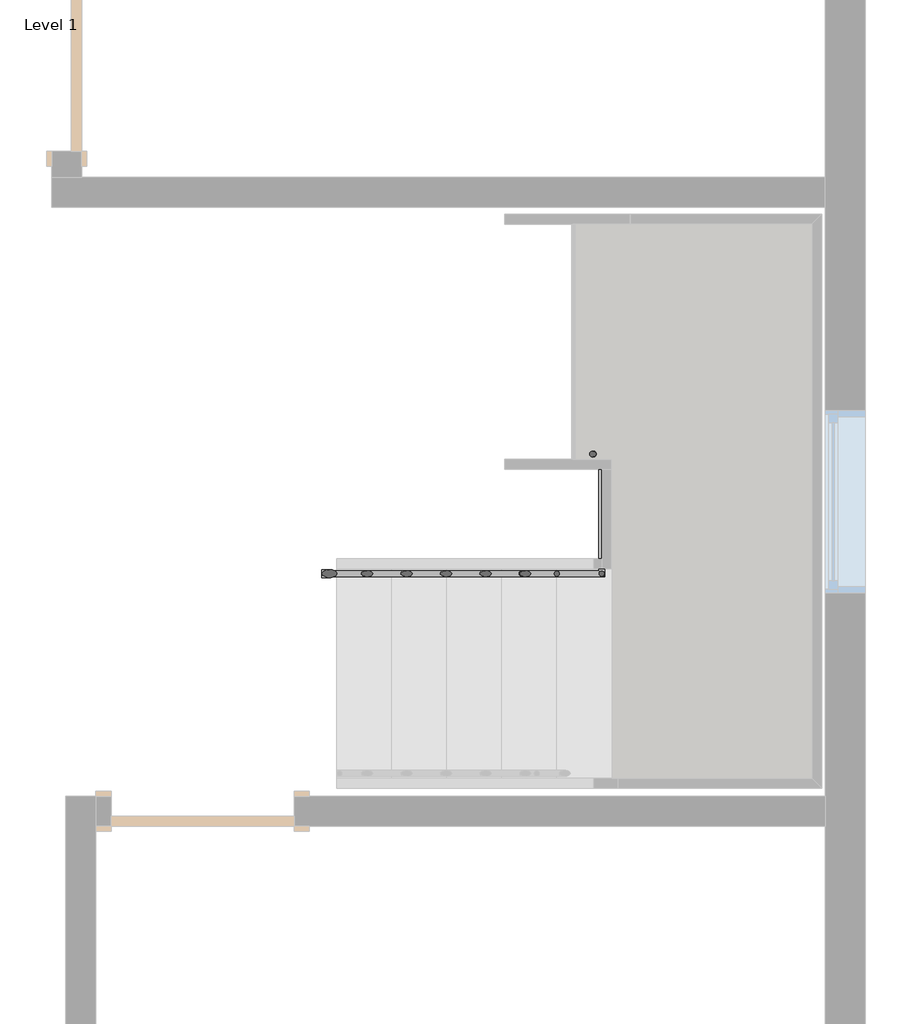
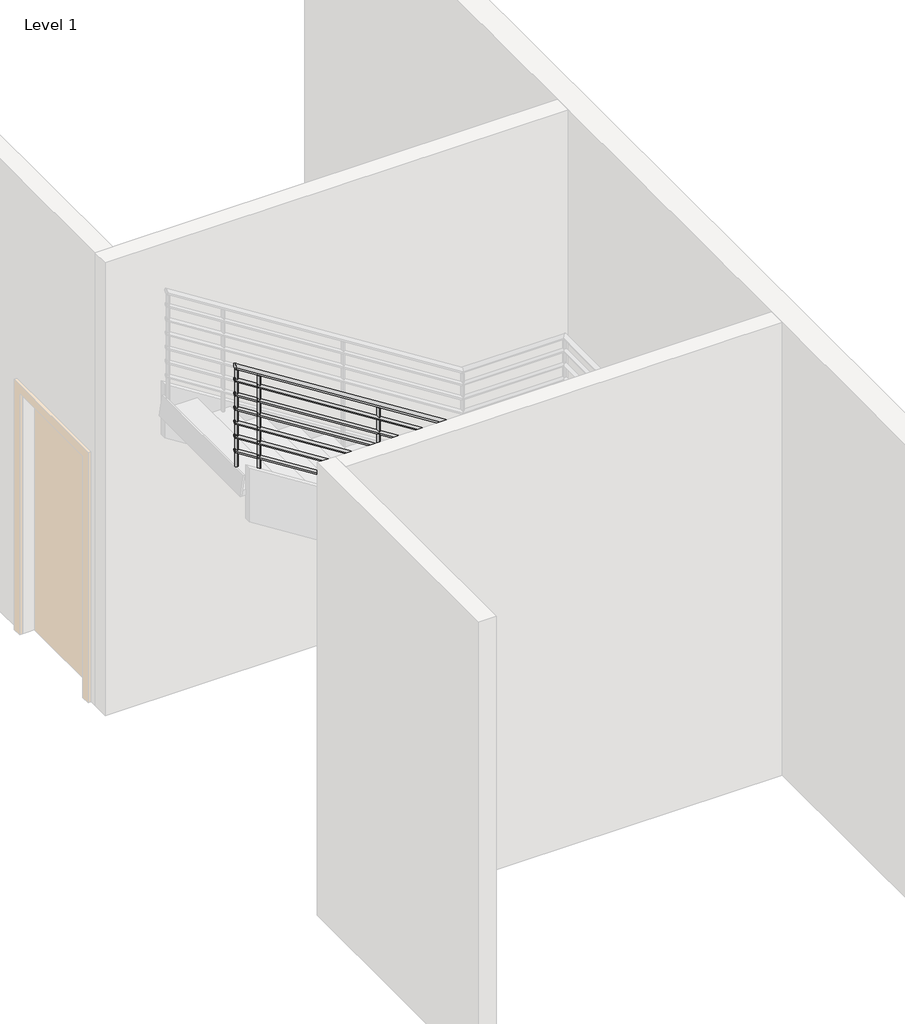
# One storey, part 2 of 3: 1 railing.
"""IFC4 building model written with IfcOpenShell, lengths in millimetres."""

from ifc_helpers import new_model, si_unit, point, frame, frame_2d, origin, place, context, project, spatial, circle_curve, ellipse_curve, trimmed, segment, composite_curve, outline, extrude, element, save
from ifc_brep_helpers import plane_surface, cylinder_surface, advanced_brep

model = new_model("IFC4")

# Units and contexts
model_context = context("Model", 3, world=origin())
ifc_project = project(units=[si_unit("LENGTHUNIT", "METRE", prefix="MILLI")], contexts=[model_context])

# Site, building, storey
site = spatial("IfcSite", under=ifc_project)
building = spatial("IfcBuilding", under=site)
storey = spatial("IfcBuildingStorey", under=building, Name="Level 1", Elevation=0.0)

# Railing
placement = place(None, origin())
element("IfcRailing", 1, ObjectType="900mm Pipe", at=placement, inside=storey, context=model_context, shape_type="SolidModel", body=[
    advanced_brep(
    [(-604.472677, 4076.0539608, 1175.9725198), (-604.472677, 4116.0539608, 1175.9725198), (577.520776, 4076.0539608, 1923.4782609), (577.520776, 4116.0539608, 1923.4782609), (815.927323, 4720.2246349, 1923.4782609), (775.927323, 4705.6846258, 1923.4782609), (775.927323, 4116.0539608, 1923.4782609), (815.927323, 4076.0539608, 1923.4782609)],
    [
        (0, 1, ellipse_curve(frame((-604.472677, 4096.0539608, 1175.9725198), z_axis=(-1.0, 0.0, 0.0), x_axis=(0.0, 0.0, -1.0)), 23.6638438, 20.0)),
        (1, 0, ellipse_curve(frame((-604.472677, 4096.0539608, 1175.9725198), z_axis=(-1.0, 0.0, 0.0), x_axis=(0.0, 0.0, -1.0)), 23.6638438, 20.0)),
        (0, 2),
        (2, 3, ellipse_curve(frame((577.520776, 4096.0539608, 1923.4782609), z_axis=(-0.9605132043335072, 0.0, -0.2782344053149755), x_axis=(0.2782344053149752, 0.0, -0.9605132043335075)), 20.822202, 20.0)),
        (3, 1),
        (3, 2, ellipse_curve(frame((577.520776, 4096.0539608, 1923.4782609), z_axis=(-0.9605132043335072, 0.0, -0.2782344053149755), x_axis=(0.2782344053149752, 0.0, -0.9605132043335075)), 20.822202, 20.0)),
        (4, 5, ellipse_curve(frame((795.927323, 4712.9546303, 1923.4782609), z_axis=(-0.25703347517711744, 0.7071067811865485, 0.6587365123009145), x_axis=(-0.25703347517712294, -0.7071067811865466, 0.6587365123009143)), 28.2842712, 20.0)),
        (5, 4, ellipse_curve(frame((795.927323, 4712.9546303, 1923.4782609), z_axis=(-0.25703347517711744, 0.7071067811865485, 0.6587365123009145), x_axis=(-0.25703347517712294, -0.7071067811865466, 0.6587365123009143)), 28.2842712, 20.0)),
        (6, 7, ellipse_curve(frame((795.927323, 4096.0539608, 1923.4782609), z_axis=(0.70710678118655, 0.707106781186545, 0.0), x_axis=(0.707106781186545, -0.70710678118655, 0.0)), 28.2842712, 20.0)),
        (7, 4),
        (5, 6),
        (7, 6, ellipse_curve(frame((795.927323, 4096.0539608, 1923.4782609), z_axis=(0.70710678118655, 0.707106781186545, 0.0), x_axis=(0.707106781186545, -0.70710678118655, 0.0)), 28.2842712, 20.0)),
        (2, 7),
        (6, 3),
    ],
    [
        plane_surface(frame((-604.472677, 4096.0539608, 1199.6363636), z_axis=(-1.0, 0.0, 0.0), x_axis=(0.0, 1.0, 0.0))),
        cylinder_surface(frame((-593.7827642, 4096.0539608, 1182.732939), z_axis=(-0.8451712313980437, 0.0, -0.5344956404098301), x_axis=(0.0, 1.0, 0.0)), 20.0),
        plane_surface(frame((795.927323, 4694.3227481, 1943.4782609), z_axis=(-0.2570334751771175, 0.7071067811865486, 0.6587365123009146), x_axis=(0.9664025003270502, 0.18806875316255517, 0.17520374266980643))),
        cylinder_surface(frame((795.927323, 4096.0539608, 1923.4782609), z_axis=(0.0, -1.0, 0.0), x_axis=(-1.0, 0.0, 0.0)), 20.0),
        cylinder_surface(frame((571.727323, 4096.0539608, 1923.4782609), z_axis=(-1.0, 0.0, 0.0), x_axis=(0.0, 1.0, 0.0)), 20.0),
    ],
    [
        (0, [[1, 2]]),
        (1, [[-1, 3, 4, 5]]),
        (1, [[-2, -5, 6, -3]]),
        (2, [[7, 8]]),
        (3, [[9, 10, -8, 11]]),
        (3, [[12, -11, -7, -10]]),
        (4, [[-4, 13, -9, 14]]),
        (4, [[-6, -14, -12, -13]]),
    ],
),
    advanced_brep(
    [(-1583.9947325, 4714.3227481, 3707.1345752), (-1583.9947325, 4674.3227481, 3707.1345752), (599.7618819, 4674.3227481, 2326.1027242), (599.7618819, 4714.3227481, 2326.1027242), (759.1654454, 4714.3227481, 1917.5763741), (744.6254363, 4674.3227481, 1954.8401385)],
    [
        (0, 1, ellipse_curve(frame((-1583.9947325, 4694.3227481, 3707.1345752), z_axis=(-1.0, 0.0, 0.0), x_axis=(0.0, 0.0, -1.0)), 23.6638438, 20.0)),
        (1, 0, ellipse_curve(frame((-1583.9947325, 4694.3227481, 3707.1345752), z_axis=(-1.0, 0.0, 0.0), x_axis=(0.0, 0.0, -1.0)), 23.6638438, 20.0)),
        (2, 3, ellipse_curve(frame((599.7618819, 4694.3227481, 2326.1027242), z_axis=(-0.636115926475422, 0.0, 0.7715934992496473), x_axis=(0.7715934992496474, 0.0, 0.6361159264754218)), 21.0517398, 20.0)),
        (3, 0),
        (1, 2),
        (3, 2, ellipse_curve(frame((599.7618819, 4694.3227481, 2326.1027242), z_axis=(-0.636115926475422, 0.0, 0.7715934992496473), x_axis=(0.7715934992496474, 0.0, 0.6361159264754218)), 21.0517398, 20.0)),
        (4, 5, ellipse_curve(frame((751.8954408, 4694.3227481, 1936.2082563), z_axis=(0.25703347517711744, -0.7071067811865485, -0.6587365123009145), x_axis=(0.25703347517712305, 0.7071067811865466, -0.6587365123009143)), 28.2842712, 20.0)),
        (5, 4, ellipse_curve(frame((751.8954408, 4694.3227481, 1936.2082563), z_axis=(0.25703347517711744, -0.7071067811865485, -0.6587365123009145), x_axis=(0.25703347517712305, 0.7071067811865466, -0.6587365123009143)), 28.2842712, 20.0)),
        (4, 3),
        (2, 5),
    ],
    [
        plane_surface(frame((-1583.9947325, 4694.3227481, 3730.798419), z_axis=(-1.0, 0.0, 0.0), x_axis=(0.0, -1.0, 0.0))),
        cylinder_surface(frame((605.3153547, 4694.3227481, 2322.5906465), z_axis=(0.8451712313980438, 0.0, -0.5344956404098301), x_axis=(0.0, -1.0, 0.0)), 20.0),
        plane_surface(frame((770.527323, 4694.3227481, 1943.4782609), z_axis=(0.2570334751771175, -0.7071067811865486, -0.6587365123009146), x_axis=(0.9664025003270502, 0.18806875316255517, 0.17520374266980643))),
        cylinder_surface(frame((751.8954408, 4694.3227481, 1936.2082563), z_axis=(0.3635002265793717, 0.0, -0.9315941097263043), x_axis=(0.0, -1.0, 0.0)), 20.0),
    ],
    [
        (0, [[1, 2]]),
        (1, [[3, 4, -2, 5]]),
        (1, [[6, -5, -1, -4]]),
        (2, [[7, 8]]),
        (3, [[-7, 9, -3, 10]]),
        (3, [[-8, -10, -6, -9]]),
    ],
),
    advanced_brep(
    [(-604.472677, 4081.0539608, 1056.8884808), (-604.472677, 4111.0539608, 1056.8884808), (576.0724128, 4081.0539608, 1803.4782609), (576.0724128, 4111.0539608, 1803.4782609), (810.927323, 4081.0539608, 1803.4782609), (780.927323, 4111.0539608, 1803.4782609), (810.927323, 4709.3227481, 1803.4782609), (780.927323, 4679.3227481, 1803.4782609), (-1583.9947325, 4709.3227481, 3588.0505361), (-1583.9947325, 4679.3227481, 3588.0505361), (603.8227283, 4679.3227481, 2204.4505609), (603.8227283, 4709.3227481, 2204.4505609), (760.2787647, 4709.3227481, 1803.4782609), (760.2787647, 4679.3227481, 1803.4782609)],
    [
        (0, 1, ellipse_curve(frame((-604.472677, 4096.0539608, 1056.8884808), z_axis=(-1.0, 0.0, 0.0), x_axis=(0.0, 0.0, -1.0)), 17.7478828, 15.0)),
        (1, 0, ellipse_curve(frame((-604.472677, 4096.0539608, 1056.8884808), z_axis=(-1.0, 0.0, 0.0), x_axis=(0.0, 0.0, -1.0)), 17.7478828, 15.0)),
        (0, 2),
        (2, 3, ellipse_curve(frame((576.0724128, 4096.0539608, 1803.4782609), z_axis=(-0.9605132043335073, 0.0, -0.2782344053149755), x_axis=(0.27823440531497556, 0.0, -0.9605132043335073)), 15.6166515, 15.0)),
        (3, 1),
        (3, 2, ellipse_curve(frame((576.0724128, 4096.0539608, 1803.4782609), z_axis=(-0.9605132043335073, 0.0, -0.2782344053149755), x_axis=(0.27823440531497556, 0.0, -0.9605132043335073)), 15.6166515, 15.0)),
        (2, 4),
        (4, 5, ellipse_curve(frame((795.927323, 4096.0539608, 1803.4782609), z_axis=(-0.70710678118655, -0.707106781186545, 0.0), x_axis=(-0.707106781186545, 0.70710678118655, 0.0)), 21.2132034, 15.0)),
        (5, 3),
        (5, 4, ellipse_curve(frame((795.927323, 4096.0539608, 1803.4782609), z_axis=(-0.70710678118655, -0.707106781186545, 0.0), x_axis=(-0.707106781186545, 0.70710678118655, 0.0)), 21.2132034, 15.0)),
        (4, 6),
        (6, 7, ellipse_curve(frame((795.927323, 4694.3227481, 1803.4782609), z_axis=(0.7071067811865449, -0.7071067811865502, 0.0), x_axis=(-0.7071067811865503, -0.7071067811865447, 0.0)), 21.2132034, 15.0)),
        (7, 5),
        (7, 6, ellipse_curve(frame((795.927323, 4694.3227481, 1803.4782609), z_axis=(0.7071067811865449, -0.7071067811865502, 0.0), x_axis=(-0.7071067811865503, -0.7071067811865447, 0.0)), 21.2132034, 15.0)),
        (8, 9, ellipse_curve(frame((-1583.9947325, 4694.3227481, 3588.0505361), z_axis=(-1.0, 0.0, 0.0), x_axis=(0.0, 0.0, -1.0)), 17.7478828, 15.0)),
        (9, 8, ellipse_curve(frame((-1583.9947325, 4694.3227481, 3588.0505361), z_axis=(-1.0, 0.0, 0.0), x_axis=(0.0, 0.0, -1.0)), 17.7478828, 15.0)),
        (10, 11, ellipse_curve(frame((603.8227283, 4694.3227481, 2204.4505609), z_axis=(-0.6361159264754221, 0.0, 0.7715934992496473), x_axis=(0.7715934992496472, 0.0, 0.6361159264754223)), 15.7888049, 15.0)),
        (11, 8),
        (9, 10),
        (11, 10, ellipse_curve(frame((603.8227283, 4694.3227481, 2204.4505609), z_axis=(-0.6361159264754221, 0.0, 0.7715934992496473), x_axis=(0.7715934992496472, 0.0, 0.6361159264754223)), 15.7888049, 15.0)),
        (6, 12),
        (12, 13, ellipse_curve(frame((760.2787647, 4694.3227481, 1803.4782609), z_axis=(0.825681605275112, 0.0, -0.5641364078929085), x_axis=(0.5641364078929086, 0.0, 0.825681605275112)), 18.166809, 15.0)),
        (13, 7),
        (13, 12, ellipse_curve(frame((760.2787647, 4694.3227481, 1803.4782609), z_axis=(0.825681605275112, 0.0, -0.5641364078929085), x_axis=(0.5641364078929086, 0.0, 0.825681605275112)), 18.166809, 15.0)),
        (12, 11),
        (10, 13),
    ],
    [
        plane_surface(frame((-604.472677, 4096.0539608, 1074.6363636), z_axis=(-1.0, 0.0, 0.0), x_axis=(0.0, 1.0, 0.0))),
        cylinder_surface(frame((-596.4552424, 4096.0539608, 1061.9587952), z_axis=(-0.8451712313980438, 0.0, -0.5344956404098301), x_axis=(0.0, 1.0, 0.0)), 15.0),
        cylinder_surface(frame((571.727323, 4096.0539608, 1803.4782609), z_axis=(-1.0, 0.0, 0.0), x_axis=(0.0, 1.0, 0.0)), 15.0),
        cylinder_surface(frame((795.927323, 4096.0539608, 1803.4782609), z_axis=(0.0, -1.0, 0.0), x_axis=(-1.0, 0.0, 0.0)), 15.0),
        plane_surface(frame((-1583.9947325, 4694.3227481, 3605.798419), z_axis=(-1.0, 0.0, 0.0), x_axis=(0.0, -1.0, 0.0))),
        cylinder_surface(frame((607.9878329, 4694.3227481, 2201.8165027), z_axis=(0.8451712313980437, 0.0, -0.53449564040983), x_axis=(0.0, -1.0, 0.0)), 15.0),
        cylinder_surface(frame((795.927323, 4694.3227481, 1803.4782609), z_axis=(1.0, 0.0, 0.0), x_axis=(0.0, -1.0, 0.0)), 15.0),
        cylinder_surface(frame((756.5534114, 4694.3227481, 1813.0257575), z_axis=(0.36350022657937175, 0.0, -0.9315941097263043), x_axis=(0.0, -1.0, 0.0)), 15.0),
    ],
    [
        (0, [[1, 2]]),
        (1, [[-1, 3, 4, 5]]),
        (1, [[-2, -5, 6, -3]]),
        (2, [[-4, 7, 8, 9]]),
        (2, [[-6, -9, 10, -7]]),
        (3, [[-8, 11, 12, 13]]),
        (3, [[-10, -13, 14, -11]]),
        (4, [[15, 16]]),
        (5, [[17, 18, -16, 19]]),
        (5, [[20, -19, -15, -18]]),
        (6, [[-12, 21, 22, 23]]),
        (6, [[-14, -23, 24, -21]]),
        (7, [[-22, 25, -17, 26]]),
        (7, [[-24, -26, -20, -25]]),
    ],
),
    advanced_brep(
    [(-604.472677, 4081.0539608, 931.8884808), (-604.472677, 4111.0539608, 931.8884808), (576.0724128, 4081.0539608, 1678.4782609), (576.0724128, 4111.0539608, 1678.4782609), (810.927323, 4081.0539608, 1678.4782609), (780.927323, 4111.0539608, 1678.4782609), (810.927323, 4709.3227481, 1678.4782609), (780.927323, 4679.3227481, 1678.4782609), (-1583.9947325, 4709.3227481, 3463.0505361), (-1583.9947325, 4679.3227481, 3463.0505361), (603.8227283, 4679.3227481, 2079.4505609), (603.8227283, 4709.3227481, 2079.4505609), (760.2787647, 4709.3227481, 1678.4782609), (760.2787647, 4679.3227481, 1678.4782609)],
    [
        (0, 1, ellipse_curve(frame((-604.472677, 4096.0539608, 931.8884808), z_axis=(-1.0, 0.0, 0.0), x_axis=(0.0, 0.0, -1.0)), 17.7478828, 15.0)),
        (1, 0, ellipse_curve(frame((-604.472677, 4096.0539608, 931.8884808), z_axis=(-1.0, 0.0, 0.0), x_axis=(0.0, 0.0, -1.0)), 17.7478828, 15.0)),
        (0, 2),
        (2, 3, ellipse_curve(frame((576.0724128, 4096.0539608, 1678.4782609), z_axis=(-0.9605132043335073, 0.0, -0.2782344053149755), x_axis=(0.27823440531497556, 0.0, -0.9605132043335073)), 15.6166515, 15.0)),
        (3, 1),
        (3, 2, ellipse_curve(frame((576.0724128, 4096.0539608, 1678.4782609), z_axis=(-0.9605132043335073, 0.0, -0.2782344053149755), x_axis=(0.27823440531497556, 0.0, -0.9605132043335073)), 15.6166515, 15.0)),
        (2, 4),
        (4, 5, ellipse_curve(frame((795.927323, 4096.0539608, 1678.4782609), z_axis=(-0.70710678118655, -0.707106781186545, 0.0), x_axis=(-0.707106781186545, 0.70710678118655, 0.0)), 21.2132034, 15.0)),
        (5, 3),
        (5, 4, ellipse_curve(frame((795.927323, 4096.0539608, 1678.4782609), z_axis=(-0.70710678118655, -0.707106781186545, 0.0), x_axis=(-0.707106781186545, 0.70710678118655, 0.0)), 21.2132034, 15.0)),
        (4, 6),
        (6, 7, ellipse_curve(frame((795.927323, 4694.3227481, 1678.4782609), z_axis=(0.7071067811865449, -0.7071067811865502, 0.0), x_axis=(-0.7071067811865503, -0.7071067811865447, 0.0)), 21.2132034, 15.0)),
        (7, 5),
        (7, 6, ellipse_curve(frame((795.927323, 4694.3227481, 1678.4782609), z_axis=(0.7071067811865449, -0.7071067811865502, 0.0), x_axis=(-0.7071067811865503, -0.7071067811865447, 0.0)), 21.2132034, 15.0)),
        (8, 9, ellipse_curve(frame((-1583.9947325, 4694.3227481, 3463.0505361), z_axis=(-1.0, 0.0, 0.0), x_axis=(0.0, 0.0, -1.0)), 17.7478828, 15.0)),
        (9, 8, ellipse_curve(frame((-1583.9947325, 4694.3227481, 3463.0505361), z_axis=(-1.0, 0.0, 0.0), x_axis=(0.0, 0.0, -1.0)), 17.7478828, 15.0)),
        (10, 11, ellipse_curve(frame((603.8227283, 4694.3227481, 2079.4505609), z_axis=(-0.636115926475422, 0.0, 0.7715934992496473), x_axis=(0.7715934992496475, 0.0, 0.6361159264754219)), 15.7888049, 15.0)),
        (11, 8),
        (9, 10),
        (11, 10, ellipse_curve(frame((603.8227283, 4694.3227481, 2079.4505609), z_axis=(-0.636115926475422, 0.0, 0.7715934992496473), x_axis=(0.7715934992496475, 0.0, 0.6361159264754219)), 15.7888049, 15.0)),
        (6, 12),
        (12, 13, ellipse_curve(frame((760.2787647, 4694.3227481, 1678.4782609), z_axis=(0.825681605275112, 0.0, -0.5641364078929085), x_axis=(0.5641364078929086, 0.0, 0.825681605275112)), 18.166809, 15.0)),
        (13, 7),
        (13, 12, ellipse_curve(frame((760.2787647, 4694.3227481, 1678.4782609), z_axis=(0.825681605275112, 0.0, -0.5641364078929085), x_axis=(0.5641364078929086, 0.0, 0.825681605275112)), 18.166809, 15.0)),
        (12, 11),
        (10, 13),
    ],
    [
        plane_surface(frame((-604.472677, 4096.0539608, 949.6363636), z_axis=(-1.0, 0.0, 0.0), x_axis=(0.0, 1.0, 0.0))),
        cylinder_surface(frame((-596.4552424, 4096.0539608, 936.9587952), z_axis=(-0.8451712313980438, 0.0, -0.5344956404098301), x_axis=(0.0, 1.0, 0.0)), 15.0),
        cylinder_surface(frame((571.727323, 4096.0539608, 1678.4782609), z_axis=(-1.0, 0.0, 0.0), x_axis=(0.0, 1.0, 0.0)), 15.0),
        cylinder_surface(frame((795.927323, 4096.0539608, 1678.4782609), z_axis=(0.0, -1.0, 0.0), x_axis=(-1.0, 0.0, 0.0)), 15.0),
        plane_surface(frame((-1583.9947325, 4694.3227481, 3480.798419), z_axis=(-1.0, 0.0, 0.0), x_axis=(0.0, -1.0, 0.0))),
        cylinder_surface(frame((607.9878329, 4694.3227481, 2076.8165027), z_axis=(0.8451712313980438, 0.0, -0.5344956404098299), x_axis=(0.0, -1.0, 0.0)), 15.0),
        cylinder_surface(frame((795.927323, 4694.3227481, 1678.4782609), z_axis=(1.0, 0.0, 0.0), x_axis=(0.0, -1.0, 0.0)), 15.0),
        cylinder_surface(frame((756.5534114, 4694.3227481, 1688.0257575), z_axis=(0.36350022657937175, 0.0, -0.9315941097263043), x_axis=(0.0, -1.0, 0.0)), 15.0),
    ],
    [
        (0, [[1, 2]]),
        (1, [[-1, 3, 4, 5]]),
        (1, [[-2, -5, 6, -3]]),
        (2, [[-4, 7, 8, 9]]),
        (2, [[-6, -9, 10, -7]]),
        (3, [[-8, 11, 12, 13]]),
        (3, [[-10, -13, 14, -11]]),
        (4, [[15, 16]]),
        (5, [[17, 18, -16, 19]]),
        (5, [[20, -19, -15, -18]]),
        (6, [[-12, 21, 22, 23]]),
        (6, [[-14, -23, 24, -21]]),
        (7, [[-22, 25, -17, 26]]),
        (7, [[-24, -26, -20, -25]]),
    ],
),
    advanced_brep(
    [(-604.472677, 4081.0539608, 806.8884808), (-604.472677, 4111.0539608, 806.8884808), (576.0724128, 4081.0539608, 1553.4782609), (576.0724128, 4111.0539608, 1553.4782609), (810.927323, 4081.0539608, 1553.4782609), (780.927323, 4111.0539608, 1553.4782609), (810.927323, 4709.3227481, 1553.4782609), (780.927323, 4679.3227481, 1553.4782609), (-1583.9947325, 4709.3227481, 3338.0505361), (-1583.9947325, 4679.3227481, 3338.0505361), (603.8227283, 4679.3227481, 1954.4505609), (603.8227283, 4709.3227481, 1954.4505609), (760.2787647, 4709.3227481, 1553.4782609), (760.2787647, 4679.3227481, 1553.4782609)],
    [
        (0, 1, ellipse_curve(frame((-604.472677, 4096.0539608, 806.8884808), z_axis=(-1.0, 0.0, 0.0), x_axis=(0.0, 0.0, -1.0)), 17.7478828, 15.0)),
        (1, 0, ellipse_curve(frame((-604.472677, 4096.0539608, 806.8884808), z_axis=(-1.0, 0.0, 0.0), x_axis=(0.0, 0.0, -1.0)), 17.7478828, 15.0)),
        (0, 2),
        (2, 3, ellipse_curve(frame((576.0724128, 4096.0539608, 1553.4782609), z_axis=(-0.9605132043335073, 0.0, -0.2782344053149755), x_axis=(0.27823440531497556, 0.0, -0.9605132043335073)), 15.6166515, 15.0)),
        (3, 1),
        (3, 2, ellipse_curve(frame((576.0724128, 4096.0539608, 1553.4782609), z_axis=(-0.9605132043335073, 0.0, -0.2782344053149755), x_axis=(0.27823440531497556, 0.0, -0.9605132043335073)), 15.6166515, 15.0)),
        (2, 4),
        (4, 5, ellipse_curve(frame((795.927323, 4096.0539608, 1553.4782609), z_axis=(-0.70710678118655, -0.707106781186545, 0.0), x_axis=(-0.707106781186545, 0.70710678118655, 0.0)), 21.2132034, 15.0)),
        (5, 3),
        (5, 4, ellipse_curve(frame((795.927323, 4096.0539608, 1553.4782609), z_axis=(-0.70710678118655, -0.707106781186545, 0.0), x_axis=(-0.707106781186545, 0.70710678118655, 0.0)), 21.2132034, 15.0)),
        (4, 6),
        (6, 7, ellipse_curve(frame((795.927323, 4694.3227481, 1553.4782609), z_axis=(0.7071067811865449, -0.7071067811865502, 0.0), x_axis=(-0.7071067811865503, -0.7071067811865447, 0.0)), 21.2132034, 15.0)),
        (7, 5),
        (7, 6, ellipse_curve(frame((795.927323, 4694.3227481, 1553.4782609), z_axis=(0.7071067811865449, -0.7071067811865502, 0.0), x_axis=(-0.7071067811865503, -0.7071067811865447, 0.0)), 21.2132034, 15.0)),
        (8, 9, ellipse_curve(frame((-1583.9947325, 4694.3227481, 3338.0505361), z_axis=(-1.0, 0.0, 0.0), x_axis=(0.0, 0.0, -1.0)), 17.7478828, 15.0)),
        (9, 8, ellipse_curve(frame((-1583.9947325, 4694.3227481, 3338.0505361), z_axis=(-1.0, 0.0, 0.0), x_axis=(0.0, 0.0, -1.0)), 17.7478828, 15.0)),
        (10, 11, ellipse_curve(frame((603.8227283, 4694.3227481, 1954.4505609), z_axis=(-0.636115926475422, 0.0, 0.7715934992496473), x_axis=(0.7715934992496475, 0.0, 0.6361159264754219)), 15.7888049, 15.0)),
        (11, 8),
        (9, 10),
        (11, 10, ellipse_curve(frame((603.8227283, 4694.3227481, 1954.4505609), z_axis=(-0.636115926475422, 0.0, 0.7715934992496473), x_axis=(0.7715934992496475, 0.0, 0.6361159264754219)), 15.7888049, 15.0)),
        (6, 12),
        (12, 13, ellipse_curve(frame((760.2787647, 4694.3227481, 1553.4782609), z_axis=(0.825681605275112, 0.0, -0.5641364078929085), x_axis=(0.5641364078929086, 0.0, 0.825681605275112)), 18.166809, 15.0)),
        (13, 7),
        (13, 12, ellipse_curve(frame((760.2787647, 4694.3227481, 1553.4782609), z_axis=(0.825681605275112, 0.0, -0.5641364078929085), x_axis=(0.5641364078929086, 0.0, 0.825681605275112)), 18.166809, 15.0)),
        (12, 11),
        (10, 13),
    ],
    [
        plane_surface(frame((-604.472677, 4096.0539608, 824.6363636), z_axis=(-1.0, 0.0, 0.0), x_axis=(0.0, 1.0, 0.0))),
        cylinder_surface(frame((-596.4552424, 4096.0539608, 811.9587952), z_axis=(-0.8451712313980438, 0.0, -0.5344956404098301), x_axis=(0.0, 1.0, 0.0)), 15.0),
        cylinder_surface(frame((571.727323, 4096.0539608, 1553.4782609), z_axis=(-1.0, 0.0, 0.0), x_axis=(0.0, 1.0, 0.0)), 15.0),
        cylinder_surface(frame((795.927323, 4096.0539608, 1553.4782609), z_axis=(0.0, -1.0, 0.0), x_axis=(-1.0, 0.0, 0.0)), 15.0),
        plane_surface(frame((-1583.9947325, 4694.3227481, 3355.798419), z_axis=(-1.0, 0.0, 0.0), x_axis=(0.0, -1.0, 0.0))),
        cylinder_surface(frame((607.9878329, 4694.3227481, 1951.8165027), z_axis=(0.8451712313980438, 0.0, -0.5344956404098299), x_axis=(0.0, -1.0, 0.0)), 15.0),
        cylinder_surface(frame((795.927323, 4694.3227481, 1553.4782609), z_axis=(1.0, 0.0, 0.0), x_axis=(0.0, -1.0, 0.0)), 15.0),
        cylinder_surface(frame((756.5534114, 4694.3227481, 1563.0257575), z_axis=(0.36350022657937175, 0.0, -0.9315941097263043), x_axis=(0.0, -1.0, 0.0)), 15.0),
    ],
    [
        (0, [[1, 2]]),
        (1, [[-1, 3, 4, 5]]),
        (1, [[-2, -5, 6, -3]]),
        (2, [[-4, 7, 8, 9]]),
        (2, [[-6, -9, 10, -7]]),
        (3, [[-8, 11, 12, 13]]),
        (3, [[-10, -13, 14, -11]]),
        (4, [[15, 16]]),
        (5, [[17, 18, -16, 19]]),
        (5, [[20, -19, -15, -18]]),
        (6, [[-12, 21, 22, 23]]),
        (6, [[-14, -23, 24, -21]]),
        (7, [[-22, 25, -17, 26]]),
        (7, [[-24, -26, -20, -25]]),
    ],
),
    advanced_brep(
    [(-604.472677, 4081.0539608, 681.8884808), (-604.472677, 4111.0539608, 681.8884808), (576.0724128, 4081.0539608, 1428.4782609), (576.0724128, 4111.0539608, 1428.4782609), (810.927323, 4081.0539608, 1428.4782609), (780.927323, 4111.0539608, 1428.4782609), (810.927323, 4709.3227481, 1428.4782609), (780.927323, 4679.3227481, 1428.4782609), (-1583.9947325, 4709.3227481, 3213.0505361), (-1583.9947325, 4679.3227481, 3213.0505361), (603.8227283, 4679.3227481, 1829.4505609), (603.8227283, 4709.3227481, 1829.4505609), (760.2787647, 4709.3227481, 1428.4782609), (760.2787647, 4679.3227481, 1428.4782609)],
    [
        (0, 1, ellipse_curve(frame((-604.472677, 4096.0539608, 681.8884808), z_axis=(-1.0, 0.0, 0.0), x_axis=(0.0, 0.0, -1.0)), 17.7478828, 15.0)),
        (1, 0, ellipse_curve(frame((-604.472677, 4096.0539608, 681.8884808), z_axis=(-1.0, 0.0, 0.0), x_axis=(0.0, 0.0, -1.0)), 17.7478828, 15.0)),
        (0, 2),
        (2, 3, ellipse_curve(frame((576.0724128, 4096.0539608, 1428.4782609), z_axis=(-0.9605132043335073, 0.0, -0.2782344053149755), x_axis=(0.27823440531497556, 0.0, -0.9605132043335073)), 15.6166515, 15.0)),
        (3, 1),
        (3, 2, ellipse_curve(frame((576.0724128, 4096.0539608, 1428.4782609), z_axis=(-0.9605132043335073, 0.0, -0.2782344053149755), x_axis=(0.27823440531497556, 0.0, -0.9605132043335073)), 15.6166515, 15.0)),
        (2, 4),
        (4, 5, ellipse_curve(frame((795.927323, 4096.0539608, 1428.4782609), z_axis=(-0.70710678118655, -0.707106781186545, 0.0), x_axis=(-0.707106781186545, 0.70710678118655, 0.0)), 21.2132034, 15.0)),
        (5, 3),
        (5, 4, ellipse_curve(frame((795.927323, 4096.0539608, 1428.4782609), z_axis=(-0.70710678118655, -0.707106781186545, 0.0), x_axis=(-0.707106781186545, 0.70710678118655, 0.0)), 21.2132034, 15.0)),
        (4, 6),
        (6, 7, ellipse_curve(frame((795.927323, 4694.3227481, 1428.4782609), z_axis=(0.7071067811865449, -0.7071067811865502, 0.0), x_axis=(-0.7071067811865503, -0.7071067811865447, 0.0)), 21.2132034, 15.0)),
        (7, 5),
        (7, 6, ellipse_curve(frame((795.927323, 4694.3227481, 1428.4782609), z_axis=(0.7071067811865449, -0.7071067811865502, 0.0), x_axis=(-0.7071067811865503, -0.7071067811865447, 0.0)), 21.2132034, 15.0)),
        (8, 9, ellipse_curve(frame((-1583.9947325, 4694.3227481, 3213.0505361), z_axis=(-1.0, 0.0, 0.0), x_axis=(0.0, 0.0, -1.0)), 17.7478828, 15.0)),
        (9, 8, ellipse_curve(frame((-1583.9947325, 4694.3227481, 3213.0505361), z_axis=(-1.0, 0.0, 0.0), x_axis=(0.0, 0.0, -1.0)), 17.7478828, 15.0)),
        (10, 11, ellipse_curve(frame((603.8227283, 4694.3227481, 1829.4505609), z_axis=(-0.636115926475422, 0.0, 0.7715934992496473), x_axis=(0.7715934992496475, 0.0, 0.6361159264754219)), 15.7888049, 15.0)),
        (11, 8),
        (9, 10),
        (11, 10, ellipse_curve(frame((603.8227283, 4694.3227481, 1829.4505609), z_axis=(-0.636115926475422, 0.0, 0.7715934992496473), x_axis=(0.7715934992496475, 0.0, 0.6361159264754219)), 15.7888049, 15.0)),
        (6, 12),
        (12, 13, ellipse_curve(frame((760.2787647, 4694.3227481, 1428.4782609), z_axis=(0.825681605275112, 0.0, -0.5641364078929085), x_axis=(0.5641364078929086, 0.0, 0.825681605275112)), 18.166809, 15.0)),
        (13, 7),
        (13, 12, ellipse_curve(frame((760.2787647, 4694.3227481, 1428.4782609), z_axis=(0.825681605275112, 0.0, -0.5641364078929085), x_axis=(0.5641364078929086, 0.0, 0.825681605275112)), 18.166809, 15.0)),
        (12, 11),
        (10, 13),
    ],
    [
        plane_surface(frame((-604.472677, 4096.0539608, 699.6363636), z_axis=(-1.0, 0.0, 0.0), x_axis=(0.0, 1.0, 0.0))),
        cylinder_surface(frame((-596.4552424, 4096.0539608, 686.9587952), z_axis=(-0.8451712313980438, 0.0, -0.5344956404098301), x_axis=(0.0, 1.0, 0.0)), 15.0),
        cylinder_surface(frame((571.727323, 4096.0539608, 1428.4782609), z_axis=(-1.0, 0.0, 0.0), x_axis=(0.0, 1.0, 0.0)), 15.0),
        cylinder_surface(frame((795.927323, 4096.0539608, 1428.4782609), z_axis=(0.0, -1.0, 0.0), x_axis=(-1.0, 0.0, 0.0)), 15.0),
        plane_surface(frame((-1583.9947325, 4694.3227481, 3230.798419), z_axis=(-1.0, 0.0, 0.0), x_axis=(0.0, -1.0, 0.0))),
        cylinder_surface(frame((607.9878329, 4694.3227481, 1826.8165027), z_axis=(0.8451712313980438, 0.0, -0.5344956404098299), x_axis=(0.0, -1.0, 0.0)), 15.0),
        cylinder_surface(frame((795.927323, 4694.3227481, 1428.4782609), z_axis=(1.0, 0.0, 0.0), x_axis=(0.0, -1.0, 0.0)), 15.0),
        cylinder_surface(frame((756.5534114, 4694.3227481, 1438.0257575), z_axis=(0.36350022657937175, 0.0, -0.9315941097263043), x_axis=(0.0, -1.0, 0.0)), 15.0),
    ],
    [
        (0, [[1, 2]]),
        (1, [[-1, 3, 4, 5]]),
        (1, [[-2, -5, 6, -3]]),
        (2, [[-4, 7, 8, 9]]),
        (2, [[-6, -9, 10, -7]]),
        (3, [[-8, 11, 12, 13]]),
        (3, [[-10, -13, 14, -11]]),
        (4, [[15, 16]]),
        (5, [[17, 18, -16, 19]]),
        (5, [[20, -19, -15, -18]]),
        (6, [[-12, 21, 22, 23]]),
        (6, [[-14, -23, 24, -21]]),
        (7, [[-22, 25, -17, 26]]),
        (7, [[-24, -26, -20, -25]]),
    ],
),
    advanced_brep(
    [(-604.472677, 4081.0539608, 556.8884808), (-604.472677, 4111.0539608, 556.8884808), (576.0724128, 4081.0539608, 1303.4782609), (576.0724128, 4111.0539608, 1303.4782609), (810.927323, 4081.0539608, 1303.4782609), (780.927323, 4111.0539608, 1303.4782609), (810.927323, 4709.3227481, 1303.4782609), (780.927323, 4679.3227481, 1303.4782609), (-1583.9947325, 4709.3227481, 3088.0505361), (-1583.9947325, 4679.3227481, 3088.0505361), (603.8227283, 4679.3227481, 1704.4505609), (603.8227283, 4709.3227481, 1704.4505609), (760.2787647, 4709.3227481, 1303.4782609), (760.2787647, 4679.3227481, 1303.4782609)],
    [
        (0, 1, ellipse_curve(frame((-604.472677, 4096.0539608, 556.8884808), z_axis=(-1.0, 0.0, 0.0), x_axis=(0.0, 0.0, -1.0)), 17.7478828, 15.0)),
        (1, 0, ellipse_curve(frame((-604.472677, 4096.0539608, 556.8884808), z_axis=(-1.0, 0.0, 0.0), x_axis=(0.0, 0.0, -1.0)), 17.7478828, 15.0)),
        (0, 2),
        (2, 3, ellipse_curve(frame((576.0724128, 4096.0539608, 1303.4782609), z_axis=(-0.9605132043335073, 0.0, -0.2782344053149755), x_axis=(0.27823440531497556, 0.0, -0.9605132043335073)), 15.6166515, 15.0)),
        (3, 1),
        (3, 2, ellipse_curve(frame((576.0724128, 4096.0539608, 1303.4782609), z_axis=(-0.9605132043335073, 0.0, -0.2782344053149755), x_axis=(0.27823440531497556, 0.0, -0.9605132043335073)), 15.6166515, 15.0)),
        (2, 4),
        (4, 5, ellipse_curve(frame((795.927323, 4096.0539608, 1303.4782609), z_axis=(-0.70710678118655, -0.707106781186545, 0.0), x_axis=(-0.707106781186545, 0.70710678118655, 0.0)), 21.2132034, 15.0)),
        (5, 3),
        (5, 4, ellipse_curve(frame((795.927323, 4096.0539608, 1303.4782609), z_axis=(-0.70710678118655, -0.707106781186545, 0.0), x_axis=(-0.707106781186545, 0.70710678118655, 0.0)), 21.2132034, 15.0)),
        (4, 6),
        (6, 7, ellipse_curve(frame((795.927323, 4694.3227481, 1303.4782609), z_axis=(0.7071067811865449, -0.7071067811865502, 0.0), x_axis=(-0.7071067811865503, -0.7071067811865447, 0.0)), 21.2132034, 15.0)),
        (7, 5),
        (7, 6, ellipse_curve(frame((795.927323, 4694.3227481, 1303.4782609), z_axis=(0.7071067811865449, -0.7071067811865502, 0.0), x_axis=(-0.7071067811865503, -0.7071067811865447, 0.0)), 21.2132034, 15.0)),
        (8, 9, ellipse_curve(frame((-1583.9947325, 4694.3227481, 3088.0505361), z_axis=(-1.0, 0.0, 0.0), x_axis=(0.0, 0.0, -1.0)), 17.7478828, 15.0)),
        (9, 8, ellipse_curve(frame((-1583.9947325, 4694.3227481, 3088.0505361), z_axis=(-1.0, 0.0, 0.0), x_axis=(0.0, 0.0, -1.0)), 17.7478828, 15.0)),
        (10, 11, ellipse_curve(frame((603.8227283, 4694.3227481, 1704.4505609), z_axis=(-0.6361159264754221, 0.0, 0.7715934992496473), x_axis=(0.7715934992496472, 0.0, 0.6361159264754223)), 15.7888049, 15.0)),
        (11, 8),
        (9, 10),
        (11, 10, ellipse_curve(frame((603.8227283, 4694.3227481, 1704.4505609), z_axis=(-0.6361159264754221, 0.0, 0.7715934992496473), x_axis=(0.7715934992496472, 0.0, 0.6361159264754223)), 15.7888049, 15.0)),
        (6, 12),
        (12, 13, ellipse_curve(frame((760.2787647, 4694.3227481, 1303.4782609), z_axis=(0.825681605275112, 0.0, -0.5641364078929085), x_axis=(0.5641364078929086, 0.0, 0.825681605275112)), 18.166809, 15.0)),
        (13, 7),
        (13, 12, ellipse_curve(frame((760.2787647, 4694.3227481, 1303.4782609), z_axis=(0.825681605275112, 0.0, -0.5641364078929085), x_axis=(0.5641364078929086, 0.0, 0.825681605275112)), 18.166809, 15.0)),
        (12, 11),
        (10, 13),
    ],
    [
        plane_surface(frame((-604.472677, 4096.0539608, 574.6363636), z_axis=(-1.0, 0.0, 0.0), x_axis=(0.0, 1.0, 0.0))),
        cylinder_surface(frame((-596.4552424, 4096.0539608, 561.9587952), z_axis=(-0.8451712313980438, 0.0, -0.5344956404098301), x_axis=(0.0, 1.0, 0.0)), 15.0),
        cylinder_surface(frame((571.727323, 4096.0539608, 1303.4782609), z_axis=(-1.0, 0.0, 0.0), x_axis=(0.0, 1.0, 0.0)), 15.0),
        cylinder_surface(frame((795.927323, 4096.0539608, 1303.4782609), z_axis=(0.0, -1.0, 0.0), x_axis=(-1.0, 0.0, 0.0)), 15.0),
        plane_surface(frame((-1583.9947325, 4694.3227481, 3105.798419), z_axis=(-1.0, 0.0, 0.0), x_axis=(0.0, -1.0, 0.0))),
        cylinder_surface(frame((607.9878329, 4694.3227481, 1701.8165027), z_axis=(0.8451712313980437, 0.0, -0.53449564040983), x_axis=(0.0, -1.0, 0.0)), 15.0),
        cylinder_surface(frame((795.927323, 4694.3227481, 1303.4782609), z_axis=(1.0, 0.0, 0.0), x_axis=(0.0, -1.0, 0.0)), 15.0),
        cylinder_surface(frame((756.5534114, 4694.3227481, 1313.0257575), z_axis=(0.36350022657937175, 0.0, -0.9315941097263043), x_axis=(0.0, -1.0, 0.0)), 15.0),
    ],
    [
        (0, [[1, 2]]),
        (1, [[-1, 3, 4, 5]]),
        (1, [[-2, -5, 6, -3]]),
        (2, [[-4, 7, 8, 9]]),
        (2, [[-6, -9, 10, -7]]),
        (3, [[-8, 11, 12, 13]]),
        (3, [[-10, -13, 14, -11]]),
        (4, [[15, 16]]),
        (5, [[17, 18, -16, 19]]),
        (5, [[20, -19, -15, -18]]),
        (6, [[-12, 21, 22, 23]]),
        (6, [[-14, -23, 24, -21]]),
        (7, [[-22, 25, -17, 26]]),
        (7, [[-24, -26, -20, -25]]),
    ],
),
    advanced_brep(
    [(-604.472677, 4081.0539608, 431.8884808), (-604.472677, 4111.0539608, 431.8884808), (576.0724128, 4081.0539608, 1178.4782609), (576.0724128, 4111.0539608, 1178.4782609), (810.927323, 4081.0539608, 1178.4782609), (780.927323, 4111.0539608, 1178.4782609), (810.927323, 4709.3227481, 1178.4782609), (780.927323, 4679.3227481, 1178.4782609), (-1583.9947325, 4709.3227481, 2963.0505361), (-1583.9947325, 4679.3227481, 2963.0505361), (603.8227283, 4679.3227481, 1579.4505609), (603.8227283, 4709.3227481, 1579.4505609), (760.2787647, 4709.3227481, 1178.4782609), (760.2787647, 4679.3227481, 1178.4782609)],
    [
        (0, 1, ellipse_curve(frame((-604.472677, 4096.0539608, 431.8884808), z_axis=(-1.0, 0.0, 0.0), x_axis=(0.0, 0.0, -1.0)), 17.7478828, 15.0)),
        (1, 0, ellipse_curve(frame((-604.472677, 4096.0539608, 431.8884808), z_axis=(-1.0, 0.0, 0.0), x_axis=(0.0, 0.0, -1.0)), 17.7478828, 15.0)),
        (0, 2),
        (2, 3, ellipse_curve(frame((576.0724128, 4096.0539608, 1178.4782609), z_axis=(-0.9605132043335073, 0.0, -0.2782344053149755), x_axis=(0.27823440531497556, 0.0, -0.9605132043335073)), 15.6166515, 15.0)),
        (3, 1),
        (3, 2, ellipse_curve(frame((576.0724128, 4096.0539608, 1178.4782609), z_axis=(-0.9605132043335073, 0.0, -0.2782344053149755), x_axis=(0.27823440531497556, 0.0, -0.9605132043335073)), 15.6166515, 15.0)),
        (2, 4),
        (4, 5, ellipse_curve(frame((795.927323, 4096.0539608, 1178.4782609), z_axis=(-0.70710678118655, -0.707106781186545, 0.0), x_axis=(-0.707106781186545, 0.70710678118655, 0.0)), 21.2132034, 15.0)),
        (5, 3),
        (5, 4, ellipse_curve(frame((795.927323, 4096.0539608, 1178.4782609), z_axis=(-0.70710678118655, -0.707106781186545, 0.0), x_axis=(-0.707106781186545, 0.70710678118655, 0.0)), 21.2132034, 15.0)),
        (4, 6),
        (6, 7, ellipse_curve(frame((795.927323, 4694.3227481, 1178.4782609), z_axis=(0.7071067811865449, -0.7071067811865502, 0.0), x_axis=(-0.7071067811865503, -0.7071067811865447, 0.0)), 21.2132034, 15.0)),
        (7, 5),
        (7, 6, ellipse_curve(frame((795.927323, 4694.3227481, 1178.4782609), z_axis=(0.7071067811865449, -0.7071067811865502, 0.0), x_axis=(-0.7071067811865503, -0.7071067811865447, 0.0)), 21.2132034, 15.0)),
        (8, 9, ellipse_curve(frame((-1583.9947325, 4694.3227481, 2963.0505361), z_axis=(-1.0, 0.0, 0.0), x_axis=(0.0, 0.0, -1.0)), 17.7478828, 15.0)),
        (9, 8, ellipse_curve(frame((-1583.9947325, 4694.3227481, 2963.0505361), z_axis=(-1.0, 0.0, 0.0), x_axis=(0.0, 0.0, -1.0)), 17.7478828, 15.0)),
        (10, 11, ellipse_curve(frame((603.8227283, 4694.3227481, 1579.4505609), z_axis=(-0.636115926475422, 0.0, 0.7715934992496473), x_axis=(0.7715934992496475, 0.0, 0.6361159264754219)), 15.7888049, 15.0)),
        (11, 8),
        (9, 10),
        (11, 10, ellipse_curve(frame((603.8227283, 4694.3227481, 1579.4505609), z_axis=(-0.636115926475422, 0.0, 0.7715934992496473), x_axis=(0.7715934992496475, 0.0, 0.6361159264754219)), 15.7888049, 15.0)),
        (6, 12),
        (12, 13, ellipse_curve(frame((760.2787647, 4694.3227481, 1178.4782609), z_axis=(0.825681605275112, 0.0, -0.5641364078929085), x_axis=(0.5641364078929086, 0.0, 0.825681605275112)), 18.166809, 15.0)),
        (13, 7),
        (13, 12, ellipse_curve(frame((760.2787647, 4694.3227481, 1178.4782609), z_axis=(0.825681605275112, 0.0, -0.5641364078929085), x_axis=(0.5641364078929086, 0.0, 0.825681605275112)), 18.166809, 15.0)),
        (12, 11),
        (10, 13),
    ],
    [
        plane_surface(frame((-604.472677, 4096.0539608, 449.6363636), z_axis=(-1.0, 0.0, 0.0), x_axis=(0.0, 1.0, 0.0))),
        cylinder_surface(frame((-596.4552424, 4096.0539608, 436.9587952), z_axis=(-0.8451712313980438, 0.0, -0.5344956404098301), x_axis=(0.0, 1.0, 0.0)), 15.0),
        cylinder_surface(frame((571.727323, 4096.0539608, 1178.4782609), z_axis=(-1.0, 0.0, 0.0), x_axis=(0.0, 1.0, 0.0)), 15.0),
        cylinder_surface(frame((795.927323, 4096.0539608, 1178.4782609), z_axis=(0.0, -1.0, 0.0), x_axis=(-1.0, 0.0, 0.0)), 15.0),
        plane_surface(frame((-1583.9947325, 4694.3227481, 2980.798419), z_axis=(-1.0, 0.0, 0.0), x_axis=(0.0, -1.0, 0.0))),
        cylinder_surface(frame((607.9878329, 4694.3227481, 1576.8165027), z_axis=(0.8451712313980438, 0.0, -0.5344956404098299), x_axis=(0.0, -1.0, 0.0)), 15.0),
        cylinder_surface(frame((795.927323, 4694.3227481, 1178.4782609), z_axis=(1.0, 0.0, 0.0), x_axis=(0.0, -1.0, 0.0)), 15.0),
        cylinder_surface(frame((756.5534114, 4694.3227481, 1188.0257575), z_axis=(0.36350022657937175, 0.0, -0.9315941097263043), x_axis=(0.0, -1.0, 0.0)), 15.0),
    ],
    [
        (0, [[1, 2]]),
        (1, [[-1, 3, 4, 5]]),
        (1, [[-2, -5, 6, -3]]),
        (2, [[-4, 7, 8, 9]]),
        (2, [[-6, -9, 10, -7]]),
        (3, [[-8, 11, 12, 13]]),
        (3, [[-10, -13, 14, -11]]),
        (4, [[15, 16]]),
        (5, [[17, 18, -16, 19]]),
        (5, [[20, -19, -15, -18]]),
        (6, [[-12, 21, 22, 23]]),
        (6, [[-14, -23, 24, -21]]),
        (7, [[-22, 25, -17, 26]]),
        (7, [[-24, -26, -20, -25]]),
    ],
),
    advanced_brep(
    [(-1383.9947325, 4681.8227481, 3556.9885179), (-1383.9947325, 4706.8227481, 3556.9885179), (-1383.9947325, 4706.8227481, 2608.6956522), (-1383.9947325, 4681.8227481, 2608.6956522)],
    [
        (0, 1, ellipse_curve(frame((-1383.9947325, 4694.3227481, 3556.9885179), z_axis=(-0.5344956404098302, 0.0, -0.8451712313980437), x_axis=(-0.8451712313980437, 0.0, 0.53449564040983)), 14.7899024, 12.5)),
        (1, 2),
        (2, 3, circle_curve(frame((-1383.9947325, 4694.3227481, 2608.6956522), z_axis=(0.0, 0.0, 1.0), x_axis=(0.0, 1.0, 0.0)), 12.5)),
        (3, 0),
        (3, 2, circle_curve(frame((-1383.9947325, 4694.3227481, 2608.6956522), z_axis=(0.0, 0.0, 1.0), x_axis=(0.0, 1.0, 0.0)), 12.5)),
        (1, 0, ellipse_curve(frame((-1383.9947325, 4694.3227481, 3556.9885179), z_axis=(-0.5344956404098302, 0.0, -0.8451712313980437), x_axis=(-0.8451712313980437, 0.0, 0.53449564040983)), 14.7899024, 12.5)),
    ],
    [
        cylinder_surface(frame((-1383.9947325, 4694.3227481, 2508.6956522), z_axis=(0.0, 0.0, 1.0), x_axis=(0.0, 1.0, 0.0)), 12.5),
        plane_surface(frame((-1408.9947325, 4719.3227481, 3572.7987946), z_axis=(0.5344956404098302, 0.0, 0.8451712313980437), x_axis=(0.0, -1.0, 0.0))),
        plane_surface(frame((-1358.9947325, 4719.3227481, 2608.6956522), z_axis=(0.0, 0.0, -1.0), x_axis=(0.0, -1.0, 0.0))),
    ],
    [
        (0, [[1, 2, 3, 4]]),
        (0, [[5, -2, 6, -4]]),
        (1, [[-6, -1]]),
        (2, [[-5, -3]]),
    ],
),
    advanced_brep(
    [(-383.9947325, 4681.8227481, 2924.5774507), (-383.9947325, 4706.8227481, 2924.5774507), (-383.9947325, 4706.8227481, 1913.0434783), (-383.9947325, 4681.8227481, 1913.0434783)],
    [
        (0, 1, ellipse_curve(frame((-383.9947325, 4694.3227481, 2924.5774507), z_axis=(-0.5344956404098302, 0.0, -0.8451712313980437), x_axis=(-0.8451712313980437, 0.0, 0.53449564040983)), 14.7899024, 12.5)),
        (1, 2),
        (2, 3, circle_curve(frame((-383.9947325, 4694.3227481, 1913.0434783), z_axis=(0.0, 0.0, 1.0), x_axis=(0.0, 1.0, 0.0)), 12.5)),
        (3, 0),
        (3, 2, circle_curve(frame((-383.9947325, 4694.3227481, 1913.0434783), z_axis=(0.0, 0.0, 1.0), x_axis=(0.0, 1.0, 0.0)), 12.5)),
        (1, 0, ellipse_curve(frame((-383.9947325, 4694.3227481, 2924.5774507), z_axis=(-0.5344956404098302, 0.0, -0.8451712313980437), x_axis=(-0.8451712313980437, 0.0, 0.53449564040983)), 14.7899024, 12.5)),
    ],
    [
        cylinder_surface(frame((-383.9947325, 4694.3227481, 1813.0434783), z_axis=(0.0, 0.0, 1.0), x_axis=(0.0, 1.0, 0.0)), 12.5),
        plane_surface(frame((-408.9947325, 4719.3227481, 2940.3877274), z_axis=(0.5344956404098302, 0.0, 0.8451712313980437), x_axis=(0.0, -1.0, 0.0))),
        plane_surface(frame((-358.9947325, 4719.3227481, 1913.0434783), z_axis=(0.0, 0.0, -1.0), x_axis=(0.0, -1.0, 0.0))),
    ],
    [
        (0, [[1, 2, 3, 4]]),
        (0, [[5, -2, 6, -4]]),
        (1, [[-6, -1]]),
        (2, [[-5, -3]]),
    ],
),
    advanced_brep(
    [(395.527323, 4108.5539608, 1784.7197432), (395.527323, 4083.5539608, 1784.7197432), (395.527323, 4083.5539608, 869.5652174), (395.527323, 4108.5539608, 869.5652174)],
    [
        (0, 1, ellipse_curve(frame((395.527323, 4096.0539608, 1784.7197432), z_axis=(0.5344956404098286, 0.0, -0.8451712313980447), x_axis=(0.8451712313980447, 0.0, 0.5344956404098286)), 14.7899024, 12.5)),
        (1, 2),
        (2, 3, circle_curve(frame((395.527323, 4096.0539608, 869.5652174), z_axis=(0.0, 0.0, 1.0), x_axis=(0.0, -1.0, 0.0)), 12.5)),
        (3, 0),
        (3, 2, circle_curve(frame((395.527323, 4096.0539608, 869.5652174), z_axis=(0.0, 0.0, 1.0), x_axis=(0.0, -1.0, 0.0)), 12.5)),
        (1, 0, ellipse_curve(frame((395.527323, 4096.0539608, 1784.7197432), z_axis=(0.5344956404098286, 0.0, -0.8451712313980447), x_axis=(0.8451712313980447, 0.0, 0.5344956404098286)), 14.7899024, 12.5)),
    ],
    [
        cylinder_surface(frame((395.527323, 4096.0539608, 769.5652174), z_axis=(0.0, 0.0, 1.0), x_axis=(0.0, -1.0, 0.0)), 12.5),
        plane_surface(frame((420.527323, 4071.0539608, 1800.5300199), z_axis=(-0.5344956404098286, 0.0, 0.8451712313980447), x_axis=(0.0, 1.0, 0.0))),
        plane_surface(frame((370.527323, 4071.0539608, 869.5652174), z_axis=(0.0, 0.0, -1.0), x_axis=(0.0, 1.0, 0.0))),
    ],
    [
        (0, [[1, 2, 3, 4]]),
        (0, [[5, -2, 6, -4]]),
        (1, [[-6, -1]]),
        (2, [[-5, -3]]),
    ],
),
    advanced_brep(
    [(616.0052675, 4681.8227481, 2229.4528743), (616.0052675, 4706.8227481, 2229.4528743), (616.0052675, 4706.8227481, 1391.3043478), (616.0052675, 4681.8227481, 1391.3043478)],
    [
        (0, 1, ellipse_curve(frame((616.0052675, 4694.3227481, 2229.4528743), z_axis=(-0.9315941097263041, 0.0, -0.36350022657937225), x_axis=(-0.3635002265793722, 0.0, 0.9315941097263039)), 34.387874, 12.5)),
        (1, 2),
        (2, 3, circle_curve(frame((616.0052675, 4694.3227481, 1391.3043478), z_axis=(0.0, 0.0, 1.0), x_axis=(0.0, 1.0, 0.0)), 12.5)),
        (3, 0),
        (3, 2, circle_curve(frame((616.0052675, 4694.3227481, 1391.3043478), z_axis=(0.0, 0.0, 1.0), x_axis=(0.0, 1.0, 0.0)), 12.5)),
        (1, 0, ellipse_curve(frame((616.0052675, 4694.3227481, 2229.4528743), z_axis=(-0.9315941097263041, 0.0, -0.36350022657937225), x_axis=(-0.3635002265793722, 0.0, 0.9315941097263039)), 34.387874, 12.5)),
    ],
    [
        cylinder_surface(frame((616.0052675, 4694.3227481, 1291.3043478), z_axis=(0.0, 0.0, 1.0), x_axis=(0.0, 1.0, 0.0)), 12.5),
        plane_surface(frame((591.0052675, 4719.3227481, 2293.523956), z_axis=(0.9315941097263041, 0.0, 0.36350022657937225), x_axis=(0.0, -1.0, 0.0))),
        plane_surface(frame((641.0052675, 4719.3227481, 1391.3043478), z_axis=(0.0, 0.0, -1.0), x_axis=(0.0, -1.0, 0.0))),
    ],
    [
        (0, [[1, 2, 3, 4]]),
        (0, [[5, -2, 6, -4]]),
        (1, [[-6, -1]]),
        (2, [[-5, -3]]),
    ],
),
    advanced_brep(
    [(770.527323, 4681.8227481, 1833.437064), (770.527323, 4706.8227481, 1833.437064), (770.527323, 4706.8227481, 1217.3913043), (770.527323, 4681.8227481, 1217.3913043)],
    [
        (0, 1, ellipse_curve(frame((770.527323, 4694.3227481, 1833.437064), z_axis=(-0.9315941097263035, 0.0, -0.3635002265793739), x_axis=(-0.3635002265793739, 0.0, 0.9315941097263034)), 34.387874, 12.5)),
        (1, 2),
        (2, 3, circle_curve(frame((770.527323, 4694.3227481, 1217.3913043), z_axis=(0.0, 0.0, 1.0), x_axis=(0.0, 1.0, 0.0)), 12.5)),
        (3, 0),
        (3, 2, circle_curve(frame((770.527323, 4694.3227481, 1217.3913043), z_axis=(0.0, 0.0, 1.0), x_axis=(0.0, 1.0, 0.0)), 12.5)),
        (1, 0, ellipse_curve(frame((770.527323, 4694.3227481, 1833.437064), z_axis=(-0.9315941097263035, 0.0, -0.3635002265793739), x_axis=(-0.3635002265793739, 0.0, 0.9315941097263034)), 34.387874, 12.5)),
    ],
    [
        cylinder_surface(frame((770.527323, 4694.3227481, 1117.3913043), z_axis=(0.0, 0.0, 1.0), x_axis=(0.0, 1.0, 0.0)), 12.5),
        plane_surface(frame((745.527323, 4719.3227481, 1897.5081458), z_axis=(0.9315941097263035, 0.0, 0.3635002265793739), x_axis=(0.0, -1.0, 0.0))),
        plane_surface(frame((795.527323, 4719.3227481, 1217.3913043), z_axis=(0.0, 0.0, -1.0), x_axis=(0.0, -1.0, 0.0))),
    ],
    [
        (0, [[1, 2, 3, 4]]),
        (0, [[5, -2, 6, -4]]),
        (1, [[-6, -1]]),
        (2, [[-5, -3]]),
    ],
),
    extrude(outline(composite_curve([segment(trimmed(circle_curve(frame_2d((795.927323, 4694.3227481)), 12.5), [point((808.427323, 4694.3227481))], [point((783.427323, 4694.3227481))], False, "CARTESIAN"), True, "CONTINUOUS"), segment(trimmed(circle_curve(frame_2d((795.927323, 4694.3227481)), 12.5), [point((783.427323, 4694.3227481))], [point((808.427323, 4694.3227481))], False, "CARTESIAN"), True, "CONTINUOUS")], self_intersect=False)), frame((0.0, 0.0, 1217.3913043), z_axis=(0.0, 0.0, 1.0), x_axis=(1.0, 0.0, 0.0)), (0.0, 0.0, 1.0), 686.0869565),
    extrude(outline(composite_curve([segment(trimmed(circle_curve(frame_2d((795.927323, 4096.0539608)), 12.5), [point((795.927323, 4083.5539608))], [point((795.927323, 4108.5539608))], False, "CARTESIAN"), True, "CONTINUOUS"), segment(trimmed(circle_curve(frame_2d((795.927323, 4096.0539608)), 12.5), [point((795.927323, 4108.5539608))], [point((795.927323, 4083.5539608))], False, "CARTESIAN"), True, "CONTINUOUS")], self_intersect=False)), frame((0.0, 0.0, 1043.4782609), z_axis=(0.0, 0.0, 1.0), x_axis=(1.0, 0.0, 0.0)), (0.0, 0.0, 1.0), 860.0),
    advanced_brep(
    [(571.727323, 4108.5539608, 1896.1505733), (571.727323, 4083.5539608, 1896.1505733), (571.727323, 4083.5539608, 1043.4782609), (571.727323, 4108.5539608, 1043.4782609)],
    [
        (0, 1, ellipse_curve(frame((571.727323, 4096.0539608, 1896.1505733), z_axis=(0.5344956404098286, 0.0, -0.8451712313980447), x_axis=(0.8451712313980447, 0.0, 0.5344956404098286)), 14.7899024, 12.5)),
        (1, 2),
        (2, 3, circle_curve(frame((571.727323, 4096.0539608, 1043.4782609), z_axis=(0.0, 0.0, 1.0), x_axis=(0.0, -1.0, 0.0)), 12.5)),
        (3, 0),
        (3, 2, circle_curve(frame((571.727323, 4096.0539608, 1043.4782609), z_axis=(0.0, 0.0, 1.0), x_axis=(0.0, -1.0, 0.0)), 12.5)),
        (1, 0, ellipse_curve(frame((571.727323, 4096.0539608, 1896.1505733), z_axis=(0.5344956404098286, 0.0, -0.8451712313980447), x_axis=(0.8451712313980447, 0.0, 0.5344956404098286)), 14.7899024, 12.5)),
    ],
    [
        cylinder_surface(frame((571.727323, 4096.0539608, 943.4782609), z_axis=(0.0, 0.0, 1.0), x_axis=(0.0, -1.0, 0.0)), 12.5),
        plane_surface(frame((596.727323, 4071.0539608, 1911.96085), z_axis=(-0.5344956404098286, 0.0, 0.8451712313980447), x_axis=(0.0, 1.0, 0.0))),
        plane_surface(frame((546.727323, 4071.0539608, 1043.4782609), z_axis=(0.0, 0.0, -1.0), x_axis=(0.0, 1.0, 0.0))),
    ],
    [
        (0, [[1, 2, 3, 4]]),
        (0, [[5, -2, 6, -4]]),
        (1, [[-6, -1]]),
        (2, [[-5, -3]]),
    ],
),
    advanced_brep(
    [(-1571.4947325, 4681.8227481, 3675.565593), (-1571.4947325, 4706.8227481, 3675.565593), (-1571.4947325, 4706.8227481, 2822.8932806), (-1571.4947325, 4681.8227481, 2822.8932806)],
    [
        (0, 1, ellipse_curve(frame((-1571.4947325, 4694.3227481, 3675.565593), z_axis=(-0.5344956404098286, 0.0, -0.8451712313980447), x_axis=(-0.8451712313980447, 0.0, 0.5344956404098286)), 14.7899024, 12.5)),
        (1, 2),
        (2, 3, circle_curve(frame((-1571.4947325, 4694.3227481, 2822.8932806), z_axis=(0.0, 0.0, 1.0), x_axis=(0.0, 1.0, 0.0)), 12.5)),
        (3, 0),
        (3, 2, circle_curve(frame((-1571.4947325, 4694.3227481, 2822.8932806), z_axis=(0.0, 0.0, 1.0), x_axis=(0.0, 1.0, 0.0)), 12.5)),
        (1, 0, ellipse_curve(frame((-1571.4947325, 4694.3227481, 3675.565593), z_axis=(-0.5344956404098286, 0.0, -0.8451712313980447), x_axis=(-0.8451712313980447, 0.0, 0.5344956404098286)), 14.7899024, 12.5)),
    ],
    [
        cylinder_surface(frame((-1571.4947325, 4694.3227481, 2722.8932806), z_axis=(0.0, 0.0, 1.0), x_axis=(0.0, 1.0, 0.0)), 12.5),
        plane_surface(frame((-1596.4947325, 4719.3227481, 3691.3758697), z_axis=(0.5344956404098286, 0.0, 0.8451712313980447), x_axis=(0.0, -1.0, 0.0))),
        plane_surface(frame((-1546.4947325, 4719.3227481, 2822.8932806), z_axis=(0.0, 0.0, -1.0), x_axis=(0.0, -1.0, 0.0))),
    ],
    [
        (0, [[1, 2, 3, 4]]),
        (0, [[5, -2, 6, -4]]),
        (1, [[-6, -1]]),
        (2, [[-5, -3]]),
    ],
),
    advanced_brep(
    [(-591.972677, 4108.5539608, 1160.2138144), (-591.972677, 4083.5539608, 1160.2138144), (-591.972677, 4083.5539608, 307.541502), (-591.972677, 4108.5539608, 307.541502)],
    [
        (0, 1, ellipse_curve(frame((-591.972677, 4096.0539608, 1160.2138144), z_axis=(0.5344956404098286, 0.0, -0.8451712313980447), x_axis=(0.8451712313980447, 0.0, 0.5344956404098286)), 14.7899024, 12.5)),
        (1, 2),
        (2, 3, circle_curve(frame((-591.972677, 4096.0539608, 307.541502), z_axis=(0.0, 0.0, 1.0), x_axis=(0.0, -1.0, 0.0)), 12.5)),
        (3, 0),
        (3, 2, circle_curve(frame((-591.972677, 4096.0539608, 307.541502), z_axis=(0.0, 0.0, 1.0), x_axis=(0.0, -1.0, 0.0)), 12.5)),
        (1, 0, ellipse_curve(frame((-591.972677, 4096.0539608, 1160.2138144), z_axis=(0.5344956404098286, 0.0, -0.8451712313980447), x_axis=(0.8451712313980447, 0.0, 0.5344956404098286)), 14.7899024, 12.5)),
    ],
    [
        cylinder_surface(frame((-591.972677, 4096.0539608, 207.541502), z_axis=(0.0, 0.0, 1.0), x_axis=(0.0, -1.0, 0.0)), 12.5),
        plane_surface(frame((-566.972677, 4071.0539608, 1176.0240911), z_axis=(-0.5344956404098286, 0.0, 0.8451712313980447), x_axis=(0.0, 1.0, 0.0))),
        plane_surface(frame((-616.972677, 4071.0539608, 307.541502), z_axis=(0.0, 0.0, -1.0), x_axis=(0.0, 1.0, 0.0))),
    ],
    [
        (0, [[1, 2, 3, 4]]),
        (0, [[5, -2, 6, -4]]),
        (1, [[-6, -1]]),
        (2, [[-5, -3]]),
    ],
),
])

save(model, "model.ifc")

# Revit data of these elements
# Type "900mm Pipe"
#   built-in parameter 1008612 = 0.019685 (stored number, unit not read)
#   built-in parameter 1008611 = 0.0984252 (stored number, unit not read)
#   built-in parameter 1008609 = 6.56168 (stored number, unit not read)
#   built-in parameter 1008604 = 0.19685 (stored number, unit not read)
#   built-in parameter 1008603 = 0.164042 (stored number, unit not read)
#   Railing Height = 900 mm
#   built-in parameter 1008630 = 2
#   built-in parameter 1008610 = 2
#   built-in parameter 1008605 = 1
#   built-in parameter 1008618 = M_Baluster - Round : 25mm
# Element 1 (IfcRailing, "900mm Pipe")
#   Phase Created = New Construction
